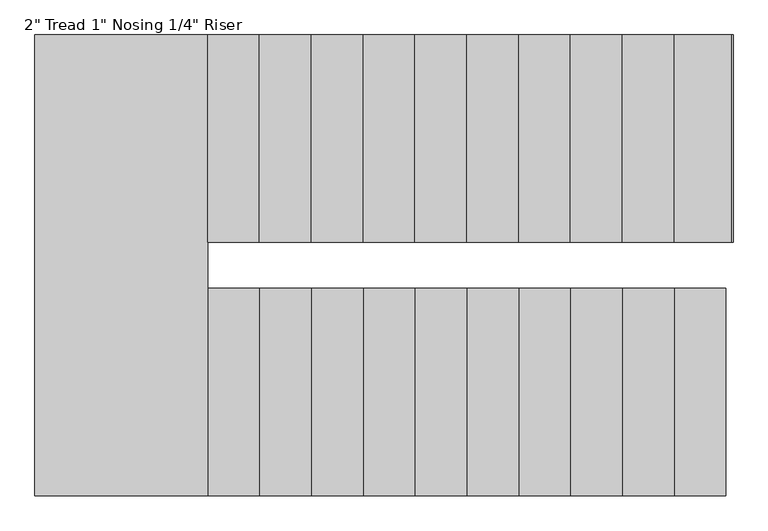
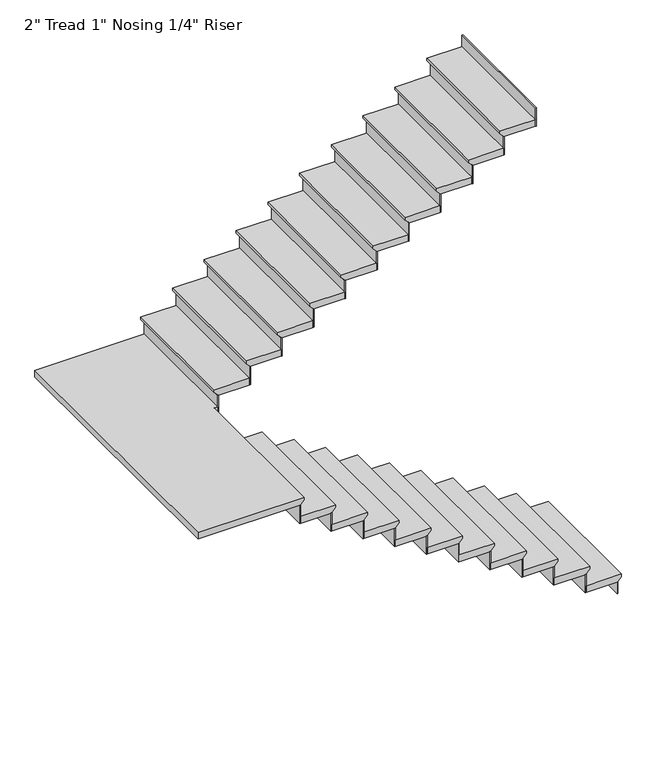
"""IFC4 building model written with IfcOpenShell, lengths in millimetres: stair flight geometry."""

from ifc_helpers import new_model, si_unit, origin, place, context, project, spatial, faceted_brep, source, transform, mapped, element, save


def stair_flight_94d610a2(model_context):
    return source(origin(), model_context, "Body", "Brep", [
        faceted_brep([(-2080.8410855, 332.1803617, 6520.2954545), (-2080.8410855, 332.1803617, 6539.3454545), (-2080.8410855, -582.2196383, 6539.3454545), (-2080.8410855, -582.2196383, 6520.2954545), (-2106.2410855, 332.1803617, 6494.8954545), (-2106.2410855, -582.2196383, 6494.8954545), (-2334.8410855, 332.1803617, 6539.3454545), (-2334.8410855, -582.2196383, 6539.3454545), (-2106.2410855, -582.2196383, 6488.5454545), (-2334.8410855, -582.2196383, 6488.5454545), (-2334.8410855, 332.1803617, 6488.5454545), (-2106.2410855, 332.1803617, 6488.5454545)], [[[0, 1, 2, 3]], [[4, 0, 3, 5]], [[2, 1, 6, 7]], [[8, 9, 10, 11]], [[2, 7, 9, 8, 5, 3]], [[8, 11, 4, 5]], [[6, 1, 0, 4, 11, 10]], [[7, 6, 10, 9]]]),
        faceted_brep([(-2106.2410855, 332.1803617, 6488.5454545), (-2106.2410855, 332.1803617, 6400.8), (-2112.5910855, 332.1803617, 6400.8), (-2112.5910855, 332.1803617, 6488.5454545), (-2106.2410855, -582.2196383, 6488.5454545), (-2112.5910855, -582.2196383, 6488.5454545), (-2112.5910855, -582.2196383, 6400.8), (-2106.2410855, -582.2196383, 6400.8)], [[[0, 1, 2, 3]], [[4, 5, 6, 7]], [[1, 0, 4, 7]], [[2, 1, 7, 6]], [[3, 2, 6, 5]], [[0, 3, 5, 4]]]),
        faceted_brep([(-2334.8410855, 332.1803617, 6627.0909091), (-2334.8410855, 332.1803617, 6488.5454545), (-2341.1910855, 332.1803617, 6488.5454545), (-2341.1910855, 332.1803617, 6627.0909091), (-2334.8410855, -582.2196383, 6627.0909091), (-2341.1910855, -582.2196383, 6627.0909091), (-2341.1910855, -582.2196383, 6488.5454545), (-2334.8410855, -582.2196383, 6488.5454545)], [[[0, 1, 2, 3]], [[4, 5, 6, 7]], [[1, 0, 4, 7]], [[2, 1, 7, 6]], [[3, 2, 6, 5]], [[0, 3, 5, 4]]]),
        faceted_brep([(-2309.4410855, -582.2196383, 6677.8909091), (-2309.4410855, 332.1803617, 6677.8909091), (-2563.4410855, 332.1803617, 6677.8909091), (-2563.4410855, -582.2196383, 6677.8909091), (-2334.8410855, -582.2196383, 6627.0909091), (-2563.4410855, -582.2196383, 6627.0909091), (-2563.4410855, 332.1803617, 6627.0909091), (-2334.8410855, 332.1803617, 6627.0909091), (-2334.8410855, -582.2196383, 6633.4409091), (-2309.4410855, -582.2196383, 6658.8409091), (-2334.8410855, 332.1803617, 6633.4409091), (-2309.4410855, 332.1803617, 6658.8409091)], [[[0, 1, 2, 3]], [[4, 5, 6, 7]], [[0, 3, 5, 4, 8, 9]], [[4, 7, 10, 8]], [[2, 1, 11, 10, 7, 6]], [[3, 2, 6, 5]], [[11, 1, 0, 9]], [[10, 11, 9, 8]]]),
        faceted_brep([(-2563.4410855, 332.1803617, 6765.6363636), (-2563.4410855, 332.1803617, 6627.0909091), (-2569.7910855, 332.1803617, 6627.0909091), (-2569.7910855, 332.1803617, 6765.6363636), (-2563.4410855, -582.2196383, 6765.6363636), (-2569.7910855, -582.2196383, 6765.6363636), (-2569.7910855, -582.2196383, 6627.0909091), (-2563.4410855, -582.2196383, 6627.0909091)], [[[0, 1, 2, 3]], [[4, 5, 6, 7]], [[1, 0, 4, 7]], [[2, 1, 7, 6]], [[3, 2, 6, 5]], [[0, 3, 5, 4]]]),
        faceted_brep([(-2538.0410855, -582.2196383, 6816.4363636), (-2538.0410855, 332.1803617, 6816.4363636), (-2792.0410855, 332.1803617, 6816.4363636), (-2792.0410855, -582.2196383, 6816.4363636), (-2563.4410855, -582.2196383, 6765.6363636), (-2792.0410855, -582.2196383, 6765.6363636), (-2792.0410855, 332.1803617, 6765.6363636), (-2563.4410855, 332.1803617, 6765.6363636), (-2563.4410855, -582.2196383, 6771.9863636), (-2538.0410855, -582.2196383, 6797.3863636), (-2563.4410855, 332.1803617, 6771.9863636), (-2538.0410855, 332.1803617, 6797.3863636)], [[[0, 1, 2, 3]], [[4, 5, 6, 7]], [[0, 3, 5, 4, 8, 9]], [[4, 7, 10, 8]], [[2, 1, 11, 10, 7, 6]], [[3, 2, 6, 5]], [[11, 1, 0, 9]], [[10, 11, 9, 8]]]),
        faceted_brep([(-2792.0410855, 332.1803617, 6904.1818182), (-2792.0410855, 332.1803617, 6765.6363636), (-2798.3910855, 332.1803617, 6765.6363636), (-2798.3910855, 332.1803617, 6904.1818182), (-2792.0410855, -582.2196383, 6904.1818182), (-2798.3910855, -582.2196383, 6904.1818182), (-2798.3910855, -582.2196383, 6765.6363636), (-2792.0410855, -582.2196383, 6765.6363636)], [[[0, 1, 2, 3]], [[4, 5, 6, 7]], [[1, 0, 4, 7]], [[2, 1, 7, 6]], [[3, 2, 6, 5]], [[0, 3, 5, 4]]]),
        faceted_brep([(-2766.6410855, -582.2196383, 6954.9818182), (-2766.6410855, 332.1803617, 6954.9818182), (-3020.6410855, 332.1803617, 6954.9818182), (-3020.6410855, -582.2196383, 6954.9818182), (-2792.0410855, -582.2196383, 6904.1818182), (-3020.6410855, -582.2196383, 6904.1818182), (-3020.6410855, 332.1803617, 6904.1818182), (-2792.0410855, 332.1803617, 6904.1818182), (-2792.0410855, -582.2196383, 6910.5318182), (-2766.6410855, -582.2196383, 6935.9318182), (-2792.0410855, 332.1803617, 6910.5318182), (-2766.6410855, 332.1803617, 6935.9318182)], [[[0, 1, 2, 3]], [[4, 5, 6, 7]], [[0, 3, 5, 4, 8, 9]], [[4, 7, 10, 8]], [[2, 1, 11, 10, 7, 6]], [[3, 2, 6, 5]], [[11, 1, 0, 9]], [[10, 11, 9, 8]]]),
        faceted_brep([(-3020.6410855, 332.1803617, 7042.7272727), (-3020.6410855, 332.1803617, 6904.1818182), (-3026.9910855, 332.1803617, 6904.1818182), (-3026.9910855, 332.1803617, 7042.7272727), (-3020.6410855, -582.2196383, 7042.7272727), (-3026.9910855, -582.2196383, 7042.7272727), (-3026.9910855, -582.2196383, 6904.1818182), (-3020.6410855, -582.2196383, 6904.1818182)], [[[0, 1, 2, 3]], [[4, 5, 6, 7]], [[1, 0, 4, 7]], [[2, 1, 7, 6]], [[3, 2, 6, 5]], [[0, 3, 5, 4]]]),
        faceted_brep([(-2995.2410855, -582.2196383, 7093.5272727), (-2995.2410855, 332.1803617, 7093.5272727), (-3249.2410855, 332.1803617, 7093.5272727), (-3249.2410855, -582.2196383, 7093.5272727), (-3020.6410855, -582.2196383, 7042.7272727), (-3249.2410855, -582.2196383, 7042.7272727), (-3249.2410855, 332.1803617, 7042.7272727), (-3020.6410855, 332.1803617, 7042.7272727), (-3020.6410855, -582.2196383, 7049.0772727), (-2995.2410855, -582.2196383, 7074.4772727), (-3020.6410855, 332.1803617, 7049.0772727), (-2995.2410855, 332.1803617, 7074.4772727)], [[[0, 1, 2, 3]], [[4, 5, 6, 7]], [[0, 3, 5, 4, 8, 9]], [[4, 7, 10, 8]], [[2, 1, 11, 10, 7, 6]], [[3, 2, 6, 5]], [[11, 1, 0, 9]], [[10, 11, 9, 8]]]),
        faceted_brep([(-3249.2410855, 332.1803617, 7181.2727273), (-3249.2410855, 332.1803617, 7042.7272727), (-3255.5910855, 332.1803617, 7042.7272727), (-3255.5910855, 332.1803617, 7181.2727273), (-3249.2410855, -582.2196383, 7181.2727273), (-3255.5910855, -582.2196383, 7181.2727273), (-3255.5910855, -582.2196383, 7042.7272727), (-3249.2410855, -582.2196383, 7042.7272727)], [[[0, 1, 2, 3]], [[4, 5, 6, 7]], [[1, 0, 4, 7]], [[2, 1, 7, 6]], [[3, 2, 6, 5]], [[0, 3, 5, 4]]]),
        faceted_brep([(-3223.8410855, -582.2196383, 7232.0727273), (-3223.8410855, 332.1803617, 7232.0727273), (-3477.8410855, 332.1803617, 7232.0727273), (-3477.8410855, -582.2196383, 7232.0727273), (-3249.2410855, -582.2196383, 7181.2727273), (-3477.8410855, -582.2196383, 7181.2727273), (-3477.8410855, 332.1803617, 7181.2727273), (-3249.2410855, 332.1803617, 7181.2727273), (-3249.2410855, -582.2196383, 7187.6227273), (-3223.8410855, -582.2196383, 7213.0227273), (-3249.2410855, 332.1803617, 7187.6227273), (-3223.8410855, 332.1803617, 7213.0227273)], [[[0, 1, 2, 3]], [[4, 5, 6, 7]], [[0, 3, 5, 4, 8, 9]], [[4, 7, 10, 8]], [[2, 1, 11, 10, 7, 6]], [[3, 2, 6, 5]], [[11, 1, 0, 9]], [[10, 11, 9, 8]]]),
        faceted_brep([(-3477.8410855, 332.1803617, 7319.8181818), (-3477.8410855, 332.1803617, 7181.2727273), (-3484.1910855, 332.1803617, 7181.2727273), (-3484.1910855, 332.1803617, 7319.8181818), (-3477.8410855, -582.2196383, 7319.8181818), (-3484.1910855, -582.2196383, 7319.8181818), (-3484.1910855, -582.2196383, 7181.2727273), (-3477.8410855, -582.2196383, 7181.2727273)], [[[0, 1, 2, 3]], [[4, 5, 6, 7]], [[1, 0, 4, 7]], [[2, 1, 7, 6]], [[3, 2, 6, 5]], [[0, 3, 5, 4]]]),
        faceted_brep([(-3452.4410855, -582.2196383, 7370.6181818), (-3452.4410855, 332.1803617, 7370.6181818), (-3706.4410855, 332.1803617, 7370.6181818), (-3706.4410855, -582.2196383, 7370.6181818), (-3477.8410855, -582.2196383, 7319.8181818), (-3706.4410855, -582.2196383, 7319.8181818), (-3706.4410855, 332.1803617, 7319.8181818), (-3477.8410855, 332.1803617, 7319.8181818), (-3477.8410855, -582.2196383, 7326.1681818), (-3452.4410855, -582.2196383, 7351.5681818), (-3477.8410855, 332.1803617, 7326.1681818), (-3452.4410855, 332.1803617, 7351.5681818)], [[[0, 1, 2, 3]], [[4, 5, 6, 7]], [[0, 3, 5, 4, 8, 9]], [[4, 7, 10, 8]], [[2, 1, 11, 10, 7, 6]], [[3, 2, 6, 5]], [[11, 1, 0, 9]], [[10, 11, 9, 8]]]),
        faceted_brep([(-3706.4410855, 332.1803617, 7458.3636364), (-3706.4410855, 332.1803617, 7319.8181818), (-3712.7910855, 332.1803617, 7319.8181818), (-3712.7910855, 332.1803617, 7458.3636364), (-3706.4410855, -582.2196383, 7458.3636364), (-3712.7910855, -582.2196383, 7458.3636364), (-3712.7910855, -582.2196383, 7319.8181818), (-3706.4410855, -582.2196383, 7319.8181818)], [[[0, 1, 2, 3]], [[4, 5, 6, 7]], [[1, 0, 4, 7]], [[2, 1, 7, 6]], [[3, 2, 6, 5]], [[0, 3, 5, 4]]]),
        faceted_brep([(-3681.0410855, -582.2196383, 7509.1636364), (-3681.0410855, 332.1803617, 7509.1636364), (-3935.0410855, 332.1803617, 7509.1636364), (-3935.0410855, -582.2196383, 7509.1636364), (-3706.4410855, -582.2196383, 7458.3636364), (-3935.0410855, -582.2196383, 7458.3636364), (-3935.0410855, 332.1803617, 7458.3636364), (-3706.4410855, 332.1803617, 7458.3636364), (-3706.4410855, -582.2196383, 7464.7136364), (-3681.0410855, -582.2196383, 7490.1136364), (-3706.4410855, 332.1803617, 7464.7136364), (-3681.0410855, 332.1803617, 7490.1136364)], [[[0, 1, 2, 3]], [[4, 5, 6, 7]], [[0, 3, 5, 4, 8, 9]], [[4, 7, 10, 8]], [[2, 1, 11, 10, 7, 6]], [[3, 2, 6, 5]], [[11, 1, 0, 9]], [[10, 11, 9, 8]]]),
        faceted_brep([(-3935.0410855, 332.1803617, 7596.9090909), (-3935.0410855, 332.1803617, 7458.3636364), (-3941.3910855, 332.1803617, 7458.3636364), (-3941.3910855, 332.1803617, 7596.9090909), (-3935.0410855, -582.2196383, 7596.9090909), (-3941.3910855, -582.2196383, 7596.9090909), (-3941.3910855, -582.2196383, 7458.3636364), (-3935.0410855, -582.2196383, 7458.3636364)], [[[0, 1, 2, 3]], [[4, 5, 6, 7]], [[1, 0, 4, 7]], [[2, 1, 7, 6]], [[3, 2, 6, 5]], [[0, 3, 5, 4]]]),
        faceted_brep([(-3909.6410855, -582.2196383, 7647.7090909), (-3909.6410855, 332.1803617, 7647.7090909), (-4163.6410855, 332.1803617, 7647.7090909), (-4163.6410855, -582.2196383, 7647.7090909), (-3935.0410855, -582.2196383, 7596.9090909), (-4163.6410855, -582.2196383, 7596.9090909), (-4163.6410855, 332.1803617, 7596.9090909), (-3935.0410855, 332.1803617, 7596.9090909), (-3935.0410855, -582.2196383, 7603.2590909), (-3909.6410855, -582.2196383, 7628.6590909), (-3935.0410855, 332.1803617, 7603.2590909), (-3909.6410855, 332.1803617, 7628.6590909)], [[[0, 1, 2, 3]], [[4, 5, 6, 7]], [[0, 3, 5, 4, 8, 9]], [[4, 7, 10, 8]], [[2, 1, 11, 10, 7, 6]], [[3, 2, 6, 5]], [[11, 1, 0, 9]], [[10, 11, 9, 8]]]),
        faceted_brep([(-4163.6410855, 332.1803617, 7735.4545455), (-4163.6410855, 332.1803617, 7596.9090909), (-4169.9910855, 332.1803617, 7596.9090909), (-4169.9910855, 332.1803617, 7735.4545455), (-4163.6410855, -582.2196383, 7735.4545455), (-4169.9910855, -582.2196383, 7735.4545455), (-4169.9910855, -582.2196383, 7596.9090909), (-4163.6410855, -582.2196383, 7596.9090909)], [[[0, 1, 2, 3]], [[4, 5, 6, 7]], [[1, 0, 4, 7]], [[2, 1, 7, 6]], [[3, 2, 6, 5]], [[0, 3, 5, 4]]]),
        faceted_brep([(-4138.2410855, -582.2196383, 7786.2545455), (-4138.2410855, 332.1803617, 7786.2545455), (-4392.2410855, 332.1803617, 7786.2545455), (-4392.2410855, -582.2196383, 7786.2545455), (-4163.6410855, -582.2196383, 7735.4545455), (-4392.2410855, -582.2196383, 7735.4545455), (-4392.2410855, 332.1803617, 7735.4545455), (-4163.6410855, 332.1803617, 7735.4545455), (-4163.6410855, -582.2196383, 7741.8045455), (-4138.2410855, -582.2196383, 7767.2045455), (-4163.6410855, 332.1803617, 7741.8045455), (-4138.2410855, 332.1803617, 7767.2045455)], [[[0, 1, 2, 3]], [[4, 5, 6, 7]], [[0, 3, 5, 4, 8, 9]], [[4, 7, 10, 8]], [[2, 1, 11, 10, 7, 6]], [[3, 2, 6, 5]], [[11, 1, 0, 9]], [[10, 11, 9, 8]]]),
        faceted_brep([(-4392.2410855, 332.1803617, 7874.0), (-4392.2410855, 332.1803617, 7735.4545455), (-4398.5910855, 332.1803617, 7735.4545455), (-4398.5910855, 332.1803617, 7874.0), (-4392.2410855, -582.2196383, 7874.0), (-4398.5910855, -582.2196383, 7874.0), (-4398.5910855, -582.2196383, 7735.4545455), (-4392.2410855, -582.2196383, 7735.4545455)], [[[0, 1, 2, 3]], [[4, 5, 6, 7]], [[1, 0, 4, 7]], [[2, 1, 7, 6]], [[3, 2, 6, 5]], [[0, 3, 5, 4]]]),
        faceted_brep([(-4341.4410855, 1449.7803617, 7924.8), (-5128.8410855, 1449.7803617, 7924.8), (-5128.8410855, -582.2196383, 7924.8), (-4366.8410855, -582.2196383, 7924.8), (-4366.8410855, 535.3803617, 7924.8), (-4341.4410855, 535.3803617, 7924.8), (-5128.8410855, 1449.7803617, 7874.0), (-4341.4410855, 1449.7803617, 7874.0), (-4341.4410855, 535.3803617, 7874.0), (-4366.8410855, 535.3803617, 7874.0), (-4366.8410855, 332.1803617, 7874.0), (-4392.2410855, 332.1803617, 7874.0), (-4392.2410855, -582.2196383, 7874.0), (-5128.8410855, -582.2196383, 7874.0), (-4392.2410855, -582.2196383, 7880.35), (-4366.8410855, -582.2196383, 7905.75), (-4392.2410855, 332.1803617, 7880.35), (-4366.8410855, 332.1803617, 7905.75)], [[[0, 1, 2, 3, 4, 5]], [[6, 7, 8, 9, 10, 11, 12, 13]], [[1, 0, 7, 6]], [[2, 1, 6, 13]], [[3, 2, 13, 12, 14, 15]], [[12, 11, 16, 14]], [[11, 10, 17, 16]], [[4, 3, 15, 17, 10, 9]], [[5, 4, 9, 8]], [[0, 5, 8, 7]], [[15, 14, 16, 17]]]),
        faceted_brep([(-4341.4410855, 535.3803617, 8012.5454545), (-4341.4410855, 535.3803617, 7874.0), (-4335.0910855, 535.3803617, 7874.0), (-4335.0910855, 535.3803617, 8012.5454545), (-4341.4410855, 1449.7803617, 8012.5454545), (-4335.0910855, 1449.7803617, 8012.5454545), (-4335.0910855, 1449.7803617, 7874.0), (-4341.4410855, 1449.7803617, 7874.0)], [[[0, 1, 2, 3]], [[4, 5, 6, 7]], [[1, 0, 4, 7]], [[2, 1, 7, 6]], [[3, 2, 6, 5]], [[0, 3, 5, 4]]]),
        faceted_brep([(-4366.8410855, 1449.7803617, 8063.3454545), (-4366.8410855, 535.3803617, 8063.3454545), (-4112.8410855, 535.3803617, 8063.3454545), (-4112.8410855, 1449.7803617, 8063.3454545), (-4341.4410855, 1449.7803617, 8012.5454545), (-4112.8410855, 1449.7803617, 8012.5454545), (-4112.8410855, 535.3803617, 8012.5454545), (-4341.4410855, 535.3803617, 8012.5454545), (-4341.4410855, 1449.7803617, 8018.8954545), (-4366.8410855, 1449.7803617, 8044.2954545), (-4341.4410855, 535.3803617, 8018.8954545), (-4366.8410855, 535.3803617, 8044.2954545)], [[[0, 1, 2, 3]], [[4, 5, 6, 7]], [[0, 3, 5, 4, 8, 9]], [[4, 7, 10, 8]], [[2, 1, 11, 10, 7, 6]], [[3, 2, 6, 5]], [[11, 1, 0, 9]], [[10, 11, 9, 8]]]),
        faceted_brep([(-4112.8410855, 535.3803617, 8151.0909091), (-4112.8410855, 535.3803617, 8012.5454545), (-4106.4910855, 535.3803617, 8012.5454545), (-4106.4910855, 535.3803617, 8151.0909091), (-4112.8410855, 1449.7803617, 8151.0909091), (-4106.4910855, 1449.7803617, 8151.0909091), (-4106.4910855, 1449.7803617, 8012.5454545), (-4112.8410855, 1449.7803617, 8012.5454545)], [[[0, 1, 2, 3]], [[4, 5, 6, 7]], [[1, 0, 4, 7]], [[2, 1, 7, 6]], [[3, 2, 6, 5]], [[0, 3, 5, 4]]]),
        faceted_brep([(-4138.2410855, 1449.7803617, 8201.8909091), (-4138.2410855, 535.3803617, 8201.8909091), (-3884.2410855, 535.3803617, 8201.8909091), (-3884.2410855, 1449.7803617, 8201.8909091), (-4112.8410855, 1449.7803617, 8151.0909091), (-3884.2410855, 1449.7803617, 8151.0909091), (-3884.2410855, 535.3803617, 8151.0909091), (-4112.8410855, 535.3803617, 8151.0909091), (-4112.8410855, 1449.7803617, 8157.4409091), (-4138.2410855, 1449.7803617, 8182.8409091), (-4112.8410855, 535.3803617, 8157.4409091), (-4138.2410855, 535.3803617, 8182.8409091)], [[[0, 1, 2, 3]], [[4, 5, 6, 7]], [[0, 3, 5, 4, 8, 9]], [[4, 7, 10, 8]], [[2, 1, 11, 10, 7, 6]], [[3, 2, 6, 5]], [[11, 1, 0, 9]], [[10, 11, 9, 8]]]),
        faceted_brep([(-3884.2410855, 535.3803617, 8289.6363636), (-3884.2410855, 535.3803617, 8151.0909091), (-3877.8910855, 535.3803617, 8151.0909091), (-3877.8910855, 535.3803617, 8289.6363636), (-3884.2410855, 1449.7803617, 8289.6363636), (-3877.8910855, 1449.7803617, 8289.6363636), (-3877.8910855, 1449.7803617, 8151.0909091), (-3884.2410855, 1449.7803617, 8151.0909091)], [[[0, 1, 2, 3]], [[4, 5, 6, 7]], [[1, 0, 4, 7]], [[2, 1, 7, 6]], [[3, 2, 6, 5]], [[0, 3, 5, 4]]]),
        faceted_brep([(-3909.6410855, 1449.7803617, 8340.4363636), (-3909.6410855, 535.3803617, 8340.4363636), (-3655.6410855, 535.3803617, 8340.4363636), (-3655.6410855, 1449.7803617, 8340.4363636), (-3884.2410855, 1449.7803617, 8289.6363636), (-3655.6410855, 1449.7803617, 8289.6363636), (-3655.6410855, 535.3803617, 8289.6363636), (-3884.2410855, 535.3803617, 8289.6363636), (-3884.2410855, 1449.7803617, 8295.9863636), (-3909.6410855, 1449.7803617, 8321.3863636), (-3884.2410855, 535.3803617, 8295.9863636), (-3909.6410855, 535.3803617, 8321.3863636)], [[[0, 1, 2, 3]], [[4, 5, 6, 7]], [[0, 3, 5, 4, 8, 9]], [[4, 7, 10, 8]], [[2, 1, 11, 10, 7, 6]], [[3, 2, 6, 5]], [[11, 1, 0, 9]], [[10, 11, 9, 8]]]),
        faceted_brep([(-3655.6410855, 535.3803617, 8428.1818182), (-3655.6410855, 535.3803617, 8289.6363636), (-3649.2910855, 535.3803617, 8289.6363636), (-3649.2910855, 535.3803617, 8428.1818182), (-3655.6410855, 1449.7803617, 8428.1818182), (-3649.2910855, 1449.7803617, 8428.1818182), (-3649.2910855, 1449.7803617, 8289.6363636), (-3655.6410855, 1449.7803617, 8289.6363636)], [[[0, 1, 2, 3]], [[4, 5, 6, 7]], [[1, 0, 4, 7]], [[2, 1, 7, 6]], [[3, 2, 6, 5]], [[0, 3, 5, 4]]]),
        faceted_brep([(-3681.0410855, 1449.7803617, 8478.9818182), (-3681.0410855, 535.3803617, 8478.9818182), (-3427.0410855, 535.3803617, 8478.9818182), (-3427.0410855, 1449.7803617, 8478.9818182), (-3655.6410855, 1449.7803617, 8428.1818182), (-3427.0410855, 1449.7803617, 8428.1818182), (-3427.0410855, 535.3803617, 8428.1818182), (-3655.6410855, 535.3803617, 8428.1818182), (-3655.6410855, 1449.7803617, 8434.5318182), (-3681.0410855, 1449.7803617, 8459.9318182), (-3655.6410855, 535.3803617, 8434.5318182), (-3681.0410855, 535.3803617, 8459.9318182)], [[[0, 1, 2, 3]], [[4, 5, 6, 7]], [[0, 3, 5, 4, 8, 9]], [[4, 7, 10, 8]], [[2, 1, 11, 10, 7, 6]], [[3, 2, 6, 5]], [[11, 1, 0, 9]], [[10, 11, 9, 8]]]),
        faceted_brep([(-3427.0410855, 535.3803617, 8566.7272727), (-3427.0410855, 535.3803617, 8428.1818182), (-3420.6910855, 535.3803617, 8428.1818182), (-3420.6910855, 535.3803617, 8566.7272727), (-3427.0410855, 1449.7803617, 8566.7272727), (-3420.6910855, 1449.7803617, 8566.7272727), (-3420.6910855, 1449.7803617, 8428.1818182), (-3427.0410855, 1449.7803617, 8428.1818182)], [[[0, 1, 2, 3]], [[4, 5, 6, 7]], [[1, 0, 4, 7]], [[2, 1, 7, 6]], [[3, 2, 6, 5]], [[0, 3, 5, 4]]]),
        faceted_brep([(-3452.4410855, 1449.7803617, 8617.5272727), (-3452.4410855, 535.3803617, 8617.5272727), (-3198.4410855, 535.3803617, 8617.5272727), (-3198.4410855, 1449.7803617, 8617.5272727), (-3427.0410855, 1449.7803617, 8566.7272727), (-3198.4410855, 1449.7803617, 8566.7272727), (-3198.4410855, 535.3803617, 8566.7272727), (-3427.0410855, 535.3803617, 8566.7272727), (-3427.0410855, 1449.7803617, 8573.0772727), (-3452.4410855, 1449.7803617, 8598.4772727), (-3427.0410855, 535.3803617, 8573.0772727), (-3452.4410855, 535.3803617, 8598.4772727)], [[[0, 1, 2, 3]], [[4, 5, 6, 7]], [[0, 3, 5, 4, 8, 9]], [[4, 7, 10, 8]], [[2, 1, 11, 10, 7, 6]], [[3, 2, 6, 5]], [[11, 1, 0, 9]], [[10, 11, 9, 8]]]),
        faceted_brep([(-3198.4410855, 535.3803617, 8705.2727273), (-3198.4410855, 535.3803617, 8566.7272727), (-3192.0910855, 535.3803617, 8566.7272727), (-3192.0910855, 535.3803617, 8705.2727273), (-3198.4410855, 1449.7803617, 8705.2727273), (-3192.0910855, 1449.7803617, 8705.2727273), (-3192.0910855, 1449.7803617, 8566.7272727), (-3198.4410855, 1449.7803617, 8566.7272727)], [[[0, 1, 2, 3]], [[4, 5, 6, 7]], [[1, 0, 4, 7]], [[2, 1, 7, 6]], [[3, 2, 6, 5]], [[0, 3, 5, 4]]]),
        faceted_brep([(-3223.8410855, 1449.7803617, 8756.0727273), (-3223.8410855, 535.3803617, 8756.0727273), (-2969.8410855, 535.3803617, 8756.0727273), (-2969.8410855, 1449.7803617, 8756.0727273), (-3198.4410855, 1449.7803617, 8705.2727273), (-2969.8410855, 1449.7803617, 8705.2727273), (-2969.8410855, 535.3803617, 8705.2727273), (-3198.4410855, 535.3803617, 8705.2727273), (-3198.4410855, 1449.7803617, 8711.6227273), (-3223.8410855, 1449.7803617, 8737.0227273), (-3198.4410855, 535.3803617, 8711.6227273), (-3223.8410855, 535.3803617, 8737.0227273)], [[[0, 1, 2, 3]], [[4, 5, 6, 7]], [[0, 3, 5, 4, 8, 9]], [[4, 7, 10, 8]], [[2, 1, 11, 10, 7, 6]], [[3, 2, 6, 5]], [[11, 1, 0, 9]], [[10, 11, 9, 8]]]),
        faceted_brep([(-2969.8410855, 535.3803617, 8843.8181818), (-2969.8410855, 535.3803617, 8705.2727273), (-2963.4910855, 535.3803617, 8705.2727273), (-2963.4910855, 535.3803617, 8843.8181818), (-2969.8410855, 1449.7803617, 8843.8181818), (-2963.4910855, 1449.7803617, 8843.8181818), (-2963.4910855, 1449.7803617, 8705.2727273), (-2969.8410855, 1449.7803617, 8705.2727273)], [[[0, 1, 2, 3]], [[4, 5, 6, 7]], [[1, 0, 4, 7]], [[2, 1, 7, 6]], [[3, 2, 6, 5]], [[0, 3, 5, 4]]]),
        faceted_brep([(-2995.2410855, 1449.7803617, 8894.6181818), (-2995.2410855, 535.3803617, 8894.6181818), (-2741.2410855, 535.3803617, 8894.6181818), (-2741.2410855, 1449.7803617, 8894.6181818), (-2969.8410855, 1449.7803617, 8843.8181818), (-2741.2410855, 1449.7803617, 8843.8181818), (-2741.2410855, 535.3803617, 8843.8181818), (-2969.8410855, 535.3803617, 8843.8181818), (-2969.8410855, 1449.7803617, 8850.1681818), (-2995.2410855, 1449.7803617, 8875.5681818), (-2969.8410855, 535.3803617, 8850.1681818), (-2995.2410855, 535.3803617, 8875.5681818)], [[[0, 1, 2, 3]], [[4, 5, 6, 7]], [[0, 3, 5, 4, 8, 9]], [[4, 7, 10, 8]], [[2, 1, 11, 10, 7, 6]], [[3, 2, 6, 5]], [[11, 1, 0, 9]], [[10, 11, 9, 8]]]),
        faceted_brep([(-2741.2410855, 535.3803617, 8982.3636364), (-2741.2410855, 535.3803617, 8843.8181818), (-2734.8910855, 535.3803617, 8843.8181818), (-2734.8910855, 535.3803617, 8982.3636364), (-2741.2410855, 1449.7803617, 8982.3636364), (-2734.8910855, 1449.7803617, 8982.3636364), (-2734.8910855, 1449.7803617, 8843.8181818), (-2741.2410855, 1449.7803617, 8843.8181818)], [[[0, 1, 2, 3]], [[4, 5, 6, 7]], [[1, 0, 4, 7]], [[2, 1, 7, 6]], [[3, 2, 6, 5]], [[0, 3, 5, 4]]]),
        faceted_brep([(-2766.6410855, 1449.7803617, 9033.1636364), (-2766.6410855, 535.3803617, 9033.1636364), (-2512.6410855, 535.3803617, 9033.1636364), (-2512.6410855, 1449.7803617, 9033.1636364), (-2741.2410855, 1449.7803617, 8982.3636364), (-2512.6410855, 1449.7803617, 8982.3636364), (-2512.6410855, 535.3803617, 8982.3636364), (-2741.2410855, 535.3803617, 8982.3636364), (-2741.2410855, 1449.7803617, 8988.7136364), (-2766.6410855, 1449.7803617, 9014.1136364), (-2741.2410855, 535.3803617, 8988.7136364), (-2766.6410855, 535.3803617, 9014.1136364)], [[[0, 1, 2, 3]], [[4, 5, 6, 7]], [[0, 3, 5, 4, 8, 9]], [[4, 7, 10, 8]], [[2, 1, 11, 10, 7, 6]], [[3, 2, 6, 5]], [[11, 1, 0, 9]], [[10, 11, 9, 8]]]),
        faceted_brep([(-2512.6410855, 535.3803617, 9120.9090909), (-2512.6410855, 535.3803617, 8982.3636364), (-2506.2910855, 535.3803617, 8982.3636364), (-2506.2910855, 535.3803617, 9120.9090909), (-2512.6410855, 1449.7803617, 9120.9090909), (-2506.2910855, 1449.7803617, 9120.9090909), (-2506.2910855, 1449.7803617, 8982.3636364), (-2512.6410855, 1449.7803617, 8982.3636364)], [[[0, 1, 2, 3]], [[4, 5, 6, 7]], [[1, 0, 4, 7]], [[2, 1, 7, 6]], [[3, 2, 6, 5]], [[0, 3, 5, 4]]]),
        faceted_brep([(-2538.0410855, 1449.7803617, 9171.7090909), (-2538.0410855, 535.3803617, 9171.7090909), (-2284.0410855, 535.3803617, 9171.7090909), (-2284.0410855, 1449.7803617, 9171.7090909), (-2512.6410855, 1449.7803617, 9120.9090909), (-2284.0410855, 1449.7803617, 9120.9090909), (-2284.0410855, 535.3803617, 9120.9090909), (-2512.6410855, 535.3803617, 9120.9090909), (-2512.6410855, 1449.7803617, 9127.2590909), (-2538.0410855, 1449.7803617, 9152.6590909), (-2512.6410855, 535.3803617, 9127.2590909), (-2538.0410855, 535.3803617, 9152.6590909)], [[[0, 1, 2, 3]], [[4, 5, 6, 7]], [[0, 3, 5, 4, 8, 9]], [[4, 7, 10, 8]], [[2, 1, 11, 10, 7, 6]], [[3, 2, 6, 5]], [[11, 1, 0, 9]], [[10, 11, 9, 8]]]),
        faceted_brep([(-2284.0410855, 535.3803617, 9259.4545455), (-2284.0410855, 535.3803617, 9120.9090909), (-2277.6910855, 535.3803617, 9120.9090909), (-2277.6910855, 535.3803617, 9259.4545455), (-2284.0410855, 1449.7803617, 9259.4545455), (-2277.6910855, 1449.7803617, 9259.4545455), (-2277.6910855, 1449.7803617, 9120.9090909), (-2284.0410855, 1449.7803617, 9120.9090909)], [[[0, 1, 2, 3]], [[4, 5, 6, 7]], [[1, 0, 4, 7]], [[2, 1, 7, 6]], [[3, 2, 6, 5]], [[0, 3, 5, 4]]]),
        faceted_brep([(-2055.4410855, 535.3803617, 9398.0), (-2055.4410855, 535.3803617, 9259.4545455), (-2049.0910855, 535.3803617, 9259.4545455), (-2049.0910855, 535.3803617, 9398.0), (-2055.4410855, 1449.7803617, 9398.0), (-2049.0910855, 1449.7803617, 9398.0), (-2049.0910855, 1449.7803617, 9259.4545455), (-2055.4410855, 1449.7803617, 9259.4545455)], [[[0, 1, 2, 3]], [[4, 5, 6, 7]], [[1, 0, 4, 7]], [[2, 1, 7, 6]], [[3, 2, 6, 5]], [[0, 3, 5, 4]]]),
        faceted_brep([(-2309.4410855, 1449.7803617, 9310.2545455), (-2309.4410855, 535.3803617, 9310.2545455), (-2055.4410855, 535.3803617, 9310.2545455), (-2055.4410855, 1449.7803617, 9310.2545455), (-2284.0410855, 1449.7803617, 9259.4545455), (-2055.4410855, 1449.7803617, 9259.4545455), (-2055.4410855, 535.3803617, 9259.4545455), (-2284.0410855, 535.3803617, 9259.4545455), (-2284.0410855, 1449.7803617, 9265.8045455), (-2309.4410855, 1449.7803617, 9291.2045455), (-2284.0410855, 535.3803617, 9265.8045455), (-2309.4410855, 535.3803617, 9291.2045455)], [[[0, 1, 2, 3]], [[4, 5, 6, 7]], [[0, 3, 5, 4, 8, 9]], [[4, 7, 10, 8]], [[2, 1, 11, 10, 7, 6]], [[3, 2, 6, 5]], [[11, 1, 0, 9]], [[10, 11, 9, 8]]]),
    ])


if __name__ == "__main__":
    model = new_model("IFC4")
    model_context = context("Model", 3, world=origin())
    ifc_project = project(units=[si_unit("LENGTHUNIT", "METRE", prefix="MILLI")], contexts=[model_context])
    site = spatial("IfcSite", under=ifc_project)
    building = spatial("IfcBuilding", under=site)
    placement = place(None, origin())
    stair_flight_shape = stair_flight_94d610a2(model_context)
    element("IfcStairFlight", 1, ObjectType="2\" Tread 1\" Nosing 1/4\" Riser", at=placement, inside=building, context=model_context, shape_type="MappedRepresentation", body=[
        mapped(stair_flight_shape, transform((0.0, 0.0, 0.0), x_axis=(1.0, 0.0, 0.0), y_axis=(0.0, 1.0, 0.0), z_axis=(0.0, 0.0, 1.0))),
    ])
    save(model, "model.ifc")
